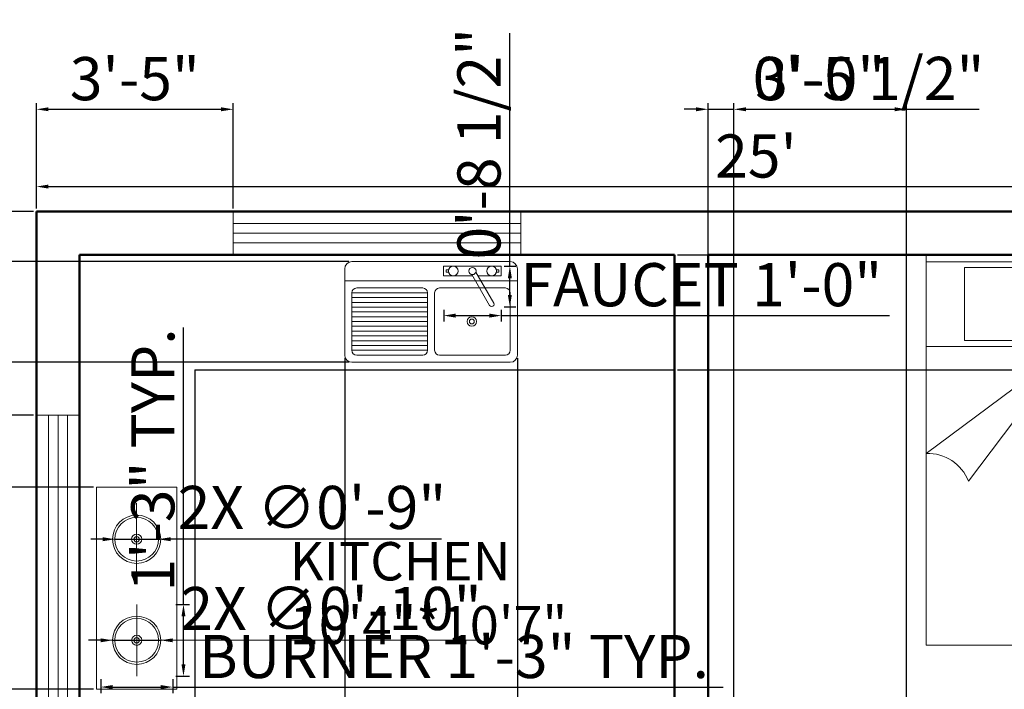
# Model space of a CAD drawing. Units: inches. Extents: x 2181 to 2717, y 1819 to 2296.
# Tile 4 of 5: x 2326 to 2531, y 2157 to 2296. Entities that reach past the tile are written whole.
import ezdxf

# ---------------------------------------------------------------- set-up
doc = ezdxf.new("R2010")
doc.units = ezdxf.units.IN
for name, color, linetype, lineweight in [('A-ANNO-DIMS', 2, 'Continuous', 13), ('A-AREA-IDEN', 7, 'Continuous', 25), ('A-EQPM', 9, 'Continuous', 18), ('A-FLOR-CASE', 32, 'Continuous', 25), ('A-FLOR-FIXT', 8, 'Continuous', 18), ('A-FURN', 8, 'Continuous', 18), ('A-GLAZ', 4, 'Continuous', 18), ('A-WALL', 7, 'Continuous', 50)]:
    doc.layers.add(name, color=color, linetype=linetype, lineweight=lineweight)
doc.styles.get("Standard").update_dxf_attribs({"font": 'arial.ttf'})
doc.dimstyles.new('ISO-25', dxfattribs={"dimtxt": 9, "dimasz": 2.5, "dimexe": 1.25, "dimexo": 0.625, "dimtad": 1, "dimlunit": 3, "dimtxsty": 'Standard', "dimcen": 2.5, "dimadec": 0, "dimazin": 0, "dimtfac": 1, "dimtmove": 0, "dimatfit": 3, "dimfxl": 1, "dimarcsym": 0})

# ---------------------------------------------------------------- blocks, each defined once
blk = doc.blocks.new('Faucet - kit sink top')
for p, q in [((-5.5, -0.75), (-5.5, -1.25)), ((-4.94278, -0.75), (-5.5, -0.75)), ((-5.5, -1.25), (-4.94278, -1.25)), ((-0.14775, -1.7441), (3.56698, -8.1782)), ((4.43301, -7.6782), (0.71828, -1.2441)), ((4.94278, -0.75), (5.5, -0.75)), ((5.5, -1.25), (4.94278, -1.25)), ((5.5, -0.75), (5.5, -1.25))]:
    blk.add_line(p, q)
blk.add_lwpolyline([(-0.00587, -2), (-6, -2), (-6, 0), (6, 0), (6, -2), (1.15195, -2)])
for centre, radius in [((-4, -1), 1), ((4, -1), 1), ((0, -1), 0.75)]:
    blk.add_circle(centre, radius)
blk.add_arc((4, -7.9282), 0.5, 210, 30)
blk = doc.blocks.new('*D8')
at = {"layer": 'A-ANNO-DIMS', "color": 0, "lineweight": -2, "transparency": 16777216}
for p, q in [((2329.35, 2256.83), (2329.35, 2262.67)), ((2629.35, 2256.83), (2629.35, 2262.67)), ((2331.85, 2261.42), (2626.85, 2261.42))]:
    blk.add_line(p, q, dxfattribs=at)
at = {"layer": 'A-ANNO-DIMS', "color": 0, "transparency": 16777216}
for points in [[(2331.85, 2261.84), (2331.85, 2261.01), (2329.35, 2261.42)], [(2626.85, 2261.84), (2626.85, 2261.01), (2629.35, 2261.42)]]:
    blk.add_solid(points, dxfattribs=at)
at = {"layer": 'Defpoints', "color": 0, "transparency": 16777216}
for p in [(2629.35, 2261.42), (2329.35, 2256.2), (2629.35, 2256.2)]:
    blk.add_point(p, dxfattribs=at)
at = {"layer": 'A-ANNO-DIMS', "color": 0, "transparency": 16777216, "insert": (2479.35, 2266.64), "char_height": 9, "attachment_point": 5}
blk.add_mtext("25'", dxfattribs=at)
blk = doc.blocks.new('WIN-60IN')
for p, q in [((0, 0), (0, 9)), ((60, 0), (60, 9)), ((60, 6.5), (0, 6.5)), ((60, 4.5), (0, 4.5)), ((60, 2.5), (0, 2.5))]:
    blk.add_line(p, q)
blk = doc.blocks.new('BED-QUEEN-PLAN')
for p, q in [((60.01, 81.47), (0, 81.47)), ((0, 81.47), (0, 80)), ((60.01, 80), (60.01, 81.47)), ((0.01, 0), (0.01, 80)), ((0.01, 80), (60.01, 80)), ((8.01, 78.8), (28.81, 78.8)), ((8.01, 63.6), (8.01, 78.8)), ((28.81, 78.8), (28.81, 63.6)), ((31.21, 78.8), (52.01, 78.8)), ((31.21, 63.6), (31.21, 78.8)), ((52.01, 78.8), (52.01, 63.6)), ((60.01, 80), (60.01, 0)), ((60.01, 62.35), (0.01, 62.35)), ((30.01, 62.35), (0.01, 40)), ((28.81, 63.6), (8.01, 63.6)), ((8.81, 34.19), (30.01, 62.35)), ((30.01, 62.35), (60.01, 40)), ((51.22, 34.19), (30.01, 62.35)), ((52.01, 63.6), (31.21, 63.6)), ((60.01, 0), (0.01, 0))]:
    blk.add_line(p, q)
for centre, start, end in [((0.34, 30.93), 21.0875, 92.0428), ((59.69, 30.93), 87.9572, 158.9125)]:
    blk.add_arc(centre, 9.08, start, end)
blk = doc.blocks.new('COOKTOP-BURNER')
for p in [(7.51, 15.01), (0, 7.51), (7.51, 0), (15.01, 7.51)]:
    blk.add_line(p, (7.51, 7.51))
for radius in [5.03, 4.55, 1.06, 0.557]:
    blk.add_circle((7.51, 7.51), radius)
blk = doc.blocks.new('*D21')
at = {"layer": 'A-ANNO-DIMS', "color": 0, "lineweight": -2, "transparency": 16777216}
for p, q in [((2342.73, 2158.61), (2342.73, 2155.73)), ((2357.74, 2158.61), (2357.74, 2155.73)), ((2345.23, 2156.98), (2355.24, 2156.98)), ((2357.74, 2156.98), (2472.54, 2156.98))]:
    blk.add_line(p, q, dxfattribs=at)
at = {"layer": 'A-ANNO-DIMS', "color": 0, "transparency": 16777216}
for points in [[(2345.23, 2157.4), (2345.23, 2156.56), (2342.73, 2156.98)], [(2355.24, 2157.4), (2355.24, 2156.56), (2357.74, 2156.98)]]:
    blk.add_solid(points, dxfattribs=at)
at = {"layer": 'Defpoints', "color": 0, "transparency": 16777216}
for p in [(2342.73, 2159.23), (2357.74, 2159.23), (2357.74, 2156.98)]:
    blk.add_point(p, dxfattribs=at)
at = {"layer": 'A-ANNO-DIMS', "color": 0, "transparency": 16777216, "insert": (2416.39, 2162.2), "char_height": 9, "attachment_point": 5}
blk.add_mtext('BURNER 1\'-3" TYP.', dxfattribs=at)
blk = doc.blocks.new('*D22')
at = {"layer": 'A-ANNO-DIMS', "color": 0, "lineweight": -2, "transparency": 16777216}
for p, q in [((2359.99, 2174.24), (2359.99, 2232.01)), ((2358.37, 2174.24), (2361.24, 2174.24)), ((2359.99, 2161.73), (2359.99, 2171.74)), ((2358.37, 2159.23), (2361.24, 2159.23))]:
    blk.add_line(p, q, dxfattribs=at)
at = {"layer": 'A-ANNO-DIMS', "color": 0, "transparency": 16777216}
for points in [[(2359.58, 2171.74), (2360.41, 2171.74), (2359.99, 2174.24)], [(2359.58, 2161.73), (2360.41, 2161.73), (2359.99, 2159.23)]]:
    blk.add_solid(points, dxfattribs=at)
at = {"layer": 'Defpoints', "color": 0, "transparency": 16777216}
for p in [(2357.74, 2174.24), (2359.99, 2174.24), (2357.74, 2159.23)]:
    blk.add_point(p, dxfattribs=at)
at = {"layer": 'A-ANNO-DIMS', "color": 0, "transparency": 16777216, "insert": (2354.77, 2204.37), "char_height": 9, "attachment_point": 5, "rotation": 90}
blk.add_mtext('1\'-3" TYP.', dxfattribs=at)
blk = doc.blocks.new('*D23')
at = {"layer": 'A-ANNO-DIMS', "color": 0, "lineweight": -2, "transparency": 16777216}
for p, q in [((2414.24, 2235.68), (2414.24, 2233.25)), ((2426.24, 2235.68), (2426.24, 2233.25)), ((2416.74, 2234.5), (2423.74, 2234.5)), ((2426.24, 2234.5), (2507.19, 2234.5))]:
    blk.add_line(p, q, dxfattribs=at)
at = {"layer": 'A-ANNO-DIMS', "color": 0, "transparency": 16777216}
for points in [[(2416.74, 2234.92), (2416.74, 2234.08), (2414.24, 2234.5)], [(2423.74, 2234.92), (2423.74, 2234.08), (2426.24, 2234.5)]]:
    blk.add_solid(points, dxfattribs=at)
at = {"layer": 'Defpoints', "color": 0, "transparency": 16777216}
for p in [(2414.24, 2236.3), (2426.24, 2236.3), (2426.24, 2234.5)]:
    blk.add_point(p, dxfattribs=at)
at = {"layer": 'A-ANNO-DIMS', "color": 0, "transparency": 16777216, "insert": (2467.96, 2239.78), "char_height": 9, "attachment_point": 5}
blk.add_mtext('FAUCET 1\'-0"', dxfattribs=at)
blk = doc.blocks.new('*D24')
at = {"layer": 'A-ANNO-DIMS', "color": 0, "lineweight": -2, "transparency": 16777216}
for p, q in [((2428.04, 2244.8), (2428.04, 2293.45)), ((2426.86, 2244.8), (2429.29, 2244.8)), ((2428.04, 2238.8), (2428.04, 2242.3)), ((2426.86, 2236.3), (2429.29, 2236.3))]:
    blk.add_line(p, q, dxfattribs=at)
at = {"layer": 'A-ANNO-DIMS', "color": 0, "transparency": 16777216}
for points in [[(2427.62, 2242.3), (2428.45, 2242.3), (2428.04, 2244.8)], [(2427.62, 2238.8), (2428.45, 2238.8), (2428.04, 2236.3)]]:
    blk.add_solid(points, dxfattribs=at)
at = {"layer": 'Defpoints', "color": 0, "transparency": 16777216}
for p in [(2426.24, 2244.8), (2428.04, 2244.8), (2426.24, 2236.3)]:
    blk.add_point(p, dxfattribs=at)
at = {"layer": 'A-ANNO-DIMS', "color": 0, "transparency": 16777216, "insert": (2422.76, 2270.37), "char_height": 9, "attachment_point": 5, "rotation": 90}
blk.add_mtext('0\'-8 1/2"', dxfattribs=at)
blk = doc.blocks.new('*D25')
at = {"layer": 'A-ANNO-DIMS', "color": 0, "lineweight": -2, "transparency": 16777216}
for p, q in [((2329.35, 2256.83), (2329.35, 2278.8)), ((2370.35, 2256.83), (2370.35, 2278.8)), ((2331.85, 2277.55), (2367.85, 2277.55))]:
    blk.add_line(p, q, dxfattribs=at)
at = {"layer": 'A-ANNO-DIMS', "color": 0, "transparency": 16777216}
for points in [[(2331.85, 2277.97), (2331.85, 2277.14), (2329.35, 2277.55)], [(2367.85, 2277.97), (2367.85, 2277.14), (2370.35, 2277.55)]]:
    blk.add_solid(points, dxfattribs=at)
at = {"layer": 'Defpoints', "color": 0, "transparency": 16777216}
for p in [(2370.35, 2277.55), (2329.35, 2256.2), (2370.35, 2256.2)]:
    blk.add_point(p, dxfattribs=at)
at = {"layer": 'A-ANNO-DIMS', "color": 0, "transparency": 16777216, "insert": (2349.85, 2282.78), "char_height": 9, "attachment_point": 5}
blk.add_mtext('3\'-5"', dxfattribs=at)
blk = doc.blocks.new('*D26')
at = {"layer": 'A-ANNO-DIMS', "color": 0, "lineweight": -2, "transparency": 16777216}
for p, q in [((2328.72, 2256.2), (2306.75, 2256.2)), ((2308, 2253.7), (2308, 2216.2)), ((2328.72, 2213.7), (2306.75, 2213.7)), ((2308, 2213.7), (2308, 2165.07))]:
    blk.add_line(p, q, dxfattribs=at)
at = {"layer": 'A-ANNO-DIMS', "color": 0, "transparency": 16777216}
for points in [[(2307.58, 2253.7), (2308.41, 2253.7), (2308, 2256.2)], [(2307.58, 2216.2), (2308.41, 2216.2), (2308, 2213.7)]]:
    blk.add_solid(points, dxfattribs=at)
at = {"layer": 'Defpoints', "color": 0, "transparency": 16777216}
for p in [(2329.35, 2256.2), (2308, 2213.7), (2329.35, 2213.7)]:
    blk.add_point(p, dxfattribs=at)
at = {"layer": 'A-ANNO-DIMS', "color": 0, "transparency": 16777216, "insert": (2302.71, 2188.13), "char_height": 9, "attachment_point": 5, "rotation": 90}
blk.add_mtext('3\'-6 1/2"', dxfattribs=at)
blk = doc.blocks.new('*D40')
at = {"layer": 'A-ANNO-DIMS', "color": 0, "lineweight": -2, "transparency": 16777216}
for p, q in [((2474.75, 2120.83), (2474.75, 2278.8)), ((2510.75, 2120.83), (2510.75, 2278.8)), ((2477.25, 2277.55), (2508.25, 2277.55))]:
    blk.add_line(p, q, dxfattribs=at)
at = {"layer": 'A-ANNO-DIMS', "color": 0, "transparency": 16777216}
for points in [[(2477.25, 2277.97), (2477.25, 2277.14), (2474.75, 2277.55)], [(2508.25, 2277.97), (2508.25, 2277.14), (2510.75, 2277.55)]]:
    blk.add_solid(points, dxfattribs=at)
at = {"layer": 'Defpoints', "color": 0, "transparency": 16777216}
for p in [(2510.75, 2277.55), (2474.75, 2120.2), (2510.75, 2120.2)]:
    blk.add_point(p, dxfattribs=at)
at = {"layer": 'A-ANNO-DIMS', "color": 0, "transparency": 16777216, "insert": (2492.75, 2282.78), "char_height": 9, "attachment_point": 5}
blk.add_mtext('3\'-0"', dxfattribs=at)
blk = doc.blocks.new('*D42')
at = {"layer": 'A-ANNO-DIMS', "color": 0, "lineweight": -2, "transparency": 16777216}
for p, q in [((2701.7, 2247.2), (2701.7, 2275.03)), ((2462.97, 2247.2), (2702.95, 2247.2)), ((2701.7, 2225.7), (2701.7, 2244.7)), ((2462.97, 2223.2), (2702.95, 2223.2))]:
    blk.add_line(p, q, dxfattribs=at)
at = {"layer": 'A-ANNO-DIMS', "color": 0, "transparency": 16777216}
for points in [[(2701.28, 2244.7), (2702.11, 2244.7), (2701.7, 2247.2)], [(2701.28, 2225.7), (2702.11, 2225.7), (2701.7, 2223.2)]]:
    blk.add_solid(points, dxfattribs=at)
at = {"layer": 'Defpoints', "color": 0, "transparency": 16777216}
for p in [(2462.35, 2247.2), (2701.7, 2247.2), (2462.35, 2223.2)]:
    blk.add_point(p, dxfattribs=at)
at = {"layer": 'A-ANNO-DIMS', "color": 0, "transparency": 16777216, "insert": (2696.48, 2262.37), "char_height": 9, "attachment_point": 5, "rotation": 90}
blk.add_mtext('2\'-0"', dxfattribs=at)
blk = doc.blocks.new('*D43')
at = {"layer": 'A-ANNO-DIMS', "color": 0, "lineweight": -2, "transparency": 16777216}
for p, q in [((2393.61, 2225.64), (2393.61, 1825.6)), ((2429.61, 2225.64), (2429.61, 1825.6)), ((2396.11, 1826.85), (2427.11, 1826.85))]:
    blk.add_line(p, q, dxfattribs=at)
at = {"layer": 'A-ANNO-DIMS', "color": 0, "transparency": 16777216}
for points in [[(2396.11, 1827.27), (2396.11, 1826.44), (2393.61, 1826.85)], [(2427.11, 1827.27), (2427.11, 1826.44), (2429.61, 1826.85)]]:
    blk.add_solid(points, dxfattribs=at)
at = {"layer": 'Defpoints', "color": 0, "transparency": 16777216}
for p in [(2393.61, 2226.26), (2429.61, 2226.26), (2429.61, 1826.85)]:
    blk.add_point(p, dxfattribs=at)
at = {"layer": 'A-ANNO-DIMS', "color": 0, "transparency": 16777216, "insert": (2411.61, 1832.08), "char_height": 9, "attachment_point": 5}
blk.add_mtext('3\'-0"', dxfattribs=at)
blk = doc.blocks.new('*D44')
at = {"layer": 'A-ANNO-DIMS', "color": 0, "lineweight": -2, "transparency": 16777216}
for p, q in [((2308, 2245.76), (2308, 2272.59)), ((2394.49, 2245.76), (2306.75, 2245.76)), ((2308, 2227.26), (2308, 2243.26)), ((2394.49, 2224.76), (2306.75, 2224.76))]:
    blk.add_line(p, q, dxfattribs=at)
at = {"layer": 'A-ANNO-DIMS', "color": 0, "transparency": 16777216}
for points in [[(2307.58, 2243.26), (2308.41, 2243.26), (2308, 2245.76)], [(2307.58, 2227.26), (2308.41, 2227.26), (2308, 2224.76)]]:
    blk.add_solid(points, dxfattribs=at)
at = {"layer": 'Defpoints', "color": 0, "transparency": 16777216}
for p in [(2308, 2245.76), (2395.11, 2245.76), (2395.11, 2224.76)]:
    blk.add_point(p, dxfattribs=at)
at = {"layer": 'A-ANNO-DIMS', "color": 0, "transparency": 16777216, "insert": (2302.78, 2260.43), "char_height": 9, "attachment_point": 5, "rotation": 90}
blk.add_mtext('1\'-9"', dxfattribs=at)
blk = doc.blocks.new('*D45')
at = {"layer": 'A-ANNO-DIMS', "color": 0, "lineweight": -2, "transparency": 16777216}
for p, q in [((2429.61, 2225.64), (2429.61, 1825.6)), ((2462.35, 2222.58), (2462.35, 1825.6)), ((2432.11, 1826.85), (2459.85, 1826.85)), ((2462.35, 1826.85), (2511.15, 1826.85))]:
    blk.add_line(p, q, dxfattribs=at)
at = {"layer": 'A-ANNO-DIMS', "color": 0, "transparency": 16777216}
for points in [[(2432.11, 1827.27), (2432.11, 1826.44), (2429.61, 1826.85)], [(2459.85, 1827.27), (2459.85, 1826.44), (2462.35, 1826.85)]]:
    blk.add_solid(points, dxfattribs=at)
at = {"layer": 'Defpoints', "color": 0, "transparency": 16777216}
for p in [(2429.61, 2226.26), (2462.35, 2223.2), (2462.35, 1826.85)]:
    blk.add_point(p, dxfattribs=at)
at = {"layer": 'A-ANNO-DIMS', "color": 0, "transparency": 16777216, "insert": (2488, 1832.13), "char_height": 9, "attachment_point": 5}
blk.add_mtext('2\'-8 1/2"', dxfattribs=at)
blk = doc.blocks.new('*D46')
at = {"layer": 'A-ANNO-DIMS', "color": 0, "lineweight": -2, "transparency": 16777216}
for p, q in [((2341.24, 2198.7), (2306.75, 2198.7)), ((2308, 2159.01), (2308, 2196.2)), ((2341.24, 2156.51), (2306.75, 2156.51))]:
    blk.add_line(p, q, dxfattribs=at)
at = {"layer": 'A-ANNO-DIMS', "color": 0, "transparency": 16777216}
for points in [[(2307.58, 2196.2), (2308.41, 2196.2), (2308, 2198.7)], [(2307.58, 2159.01), (2308.41, 2159.01), (2308, 2156.51)]]:
    blk.add_solid(points, dxfattribs=at)
at = {"layer": 'Defpoints', "color": 0, "transparency": 16777216}
for p in [(2308, 2198.7), (2341.86, 2198.7), (2341.86, 2156.51)]:
    blk.add_point(p, dxfattribs=at)
at = {"layer": 'A-ANNO-DIMS', "color": 0, "transparency": 16777216, "insert": (2302.77, 2177.61), "char_height": 9, "attachment_point": 5, "rotation": 90}
blk.add_mtext('3\'-6"', dxfattribs=at)
blk = doc.blocks.new('*D48')
at = {"layer": 'A-ANNO-DIMS', "color": 0, "lineweight": -2, "transparency": 16777216}
for p, q in [((2308, 2156.51), (2308, 2205.15)), ((2341.24, 2156.51), (2306.75, 2156.51)), ((2308, 2122.7), (2308, 2154.01)), ((2337.72, 2120.2), (2306.75, 2120.2))]:
    blk.add_line(p, q, dxfattribs=at)
at = {"layer": 'A-ANNO-DIMS', "color": 0, "transparency": 16777216}
for points in [[(2307.58, 2154.01), (2308.41, 2154.01), (2308, 2156.51)], [(2307.58, 2122.7), (2308.41, 2122.7), (2308, 2120.2)]]:
    blk.add_solid(points, dxfattribs=at)
at = {"layer": 'Defpoints', "color": 0, "transparency": 16777216}
for p in [(2308, 2156.51), (2341.86, 2156.51), (2338.35, 2120.2)]:
    blk.add_point(p, dxfattribs=at)
at = {"layer": 'A-ANNO-DIMS', "color": 0, "transparency": 16777216, "insert": (2302.71, 2182.08), "char_height": 9, "attachment_point": 5, "rotation": 90}
blk.add_mtext('3\'-0 1/2"', dxfattribs=at)
blk = doc.blocks.new('*D61')
at = {"layer": 'A-ANNO-DIMS', "color": 0, "lineweight": -2, "transparency": 16777216}
for p, q in [((2469.35, 2120.83), (2469.35, 2278.8)), ((2474.75, 2120.83), (2474.75, 2278.8)), ((2466.85, 2277.55), (2464.35, 2277.55)), ((2469.35, 2277.55), (2474.75, 2277.55)), ((2477.25, 2277.55), (2525.9, 2277.55))]:
    blk.add_line(p, q, dxfattribs=at)
at = {"layer": 'A-ANNO-DIMS', "color": 0, "transparency": 16777216}
for points in [[(2466.85, 2277.97), (2466.85, 2277.14), (2469.35, 2277.55)], [(2477.25, 2277.97), (2477.25, 2277.14), (2474.75, 2277.55)]]:
    blk.add_solid(points, dxfattribs=at)
at = {"layer": 'Defpoints', "color": 0, "transparency": 16777216}
for p in [(2474.75, 2277.55), (2469.35, 2120.2), (2474.75, 2120.2)]:
    blk.add_point(p, dxfattribs=at)
at = {"layer": 'A-ANNO-DIMS', "color": 0, "transparency": 16777216, "insert": (2502.82, 2282.83), "char_height": 9, "attachment_point": 5}
blk.add_mtext('0\'-5 1/2"', dxfattribs=at)
blk = doc.blocks.new('*D63')
at = {"layer": 'A-ANNO-DIMS', "color": 0, "lineweight": -2, "transparency": 16777216}
for p, q in [((2342.7, 2166.74), (2340.2, 2166.74)), ((2345.2, 2166.74), (2355.27, 2166.74)), ((2421.24, 2166.73), (2357.77, 2166.74))]:
    blk.add_line(p, q, dxfattribs=at)
at = {"layer": 'A-ANNO-DIMS', "color": 0, "transparency": 16777216}
for points in [[(2342.7, 2167.15), (2342.7, 2166.32), (2345.2, 2166.74)], [(2357.77, 2167.15), (2357.77, 2166.32), (2355.27, 2166.74)]]:
    blk.add_solid(points, dxfattribs=at)
at = {"layer": 'Defpoints', "color": 0, "transparency": 16777216}
for p in [(2345.2, 2166.74), (2355.27, 2166.74)]:
    blk.add_point(p, dxfattribs=at)
at = {"layer": 'A-ANNO-DIMS', "color": 0, "transparency": 16777216, "insert": (2390.75, 2172.21), "char_height": 9, "attachment_point": 5, "rotation": 359.9974}
blk.add_mtext('2X ∅0\'-10"', dxfattribs=at)
blk = doc.blocks.new('*D64')
at = {"layer": 'A-ANNO-DIMS', "color": 0, "lineweight": -2, "transparency": 16777216}
for p, q in [((2343.18, 2187.83), (2340.68, 2187.83)), ((2345.68, 2187.83), (2354.79, 2187.83)), ((2413.77, 2187.83), (2357.29, 2187.83))]:
    blk.add_line(p, q, dxfattribs=at)
at = {"layer": 'A-ANNO-DIMS', "color": 0, "transparency": 16777216}
for points in [[(2343.18, 2188.25), (2343.18, 2187.42), (2345.68, 2187.83)], [(2357.29, 2188.25), (2357.29, 2187.42), (2354.79, 2187.83)]]:
    blk.add_solid(points, dxfattribs=at)
at = {"layer": 'Defpoints', "color": 0, "transparency": 16777216}
for p in [(2345.68, 2187.83), (2354.79, 2187.83)]:
    blk.add_point(p, dxfattribs=at)
at = {"layer": 'A-ANNO-DIMS', "color": 0, "transparency": 16777216, "insert": (2386.78, 2193.3), "char_height": 9, "attachment_point": 5, "rotation": 359.9974}
blk.add_mtext('2X ∅0\'-9"', dxfattribs=at)

msp = doc.modelspace()

# ---------------------------------------------------------------- linework, layer by layer
at = {"layer": 'A-EQPM'}
msp.add_lwpolyline([(2341.861, 2198.704), (2358.609, 2198.704), (2358.609, 2156.51), (2341.861, 2156.51)], close=True, dxfattribs=at)
at = {"layer": 'A-FLOR-CASE'}
for q in [(2362.346, 2120.205), (2462.346, 2223.205)]:
    msp.add_line((2362.346, 2223.205), q, dxfattribs=at)
at = {"layer": 'A-FLOR-FIXT'}
for p, q in [((2393.61, 2241.763), (2429.61, 2241.763)), ((2410.86, 2227.263), (2410.86, 2239.263)), ((2412.36, 2239.263), (2412.36, 2227.263)), ((2396.11, 2226.263), (2409.86, 2226.263))]:
    msp.add_line(p, q, dxfattribs=at)
for points in [[(2395.11, 2245.763), (2428.11, 2245.763)], [(2393.61, 2226.263), (2393.61, 2244.263)], [(2429.61, 2244.263), (2429.61, 2226.263)], [(2396.11, 2240.263), (2409.86, 2240.263)], [(2413.36, 2240.263), (2427.11, 2240.263)], [(2395.11, 2227.263), (2395.11, 2239.263)], [(2395.11, 2239.263), (2410.86, 2239.263)], [(2395.11, 2238.263), (2410.86, 2238.263)], [(2428.11, 2239.263), (2428.11, 2227.263)], [(2395.11, 2237.263), (2410.86, 2237.263)], [(2395.11, 2236.263), (2410.86, 2236.263)], [(2395.11, 2235.263), (2410.86, 2235.263)], [(2395.11, 2234.263), (2410.86, 2234.263)], [(2395.11, 2233.263), (2410.86, 2233.263)], [(2395.11, 2232.263), (2410.86, 2232.263)], [(2395.11, 2231.263), (2410.86, 2231.263)], [(2395.11, 2230.263), (2410.86, 2230.263)], [(2395.11, 2229.263), (2410.86, 2229.263)], [(2395.11, 2228.263), (2410.86, 2228.263)], [(2395.11, 2227.263), (2410.86, 2227.263)], [(2427.11, 2226.263), (2413.36, 2226.263)], [(2428.11, 2224.763), (2395.11, 2224.763)]]:
    msp.add_lwpolyline(points, dxfattribs=at)
for radius in [1, 0.5]:
    msp.add_circle((2420.11, 2233.263), radius, dxfattribs=at)
for centre, radius, start, end in [((2395.11, 2244.263), 1.5, 90, 180), ((2428.11, 2244.263), 1.5, 0, 90), ((2396.11, 2239.263), 1, 90, 180), ((2409.86, 2239.263), 1, 0, 90), ((2413.36, 2239.263), 1, 90, 180), ((2427.11, 2239.263), 1, 0, 90), ((2396.11, 2227.263), 1, 180, 270), ((2409.86, 2227.263), 1, 270, 0), ((2413.36, 2227.263), 1, 180, 270), ((2427.11, 2227.263), 1, 270, 0), ((2395.11, 2226.263), 1.5, 180, 270), ((2428.11, 2226.263), 1.5, 270, 0)]:
    msp.add_arc(centre, radius, start, end, dxfattribs=at)
at = {"layer": 'A-WALL'}
for p, q in [((2329.346, 2256.205), (2629.346, 2256.205)), ((2329.346, 2256.205), (2329.346, 1872.205)), ((2338.346, 2247.205), (2462.346, 2247.205)), ((2338.346, 2247.205), (2338.346, 2120.205)), ((2462.346, 2247.205), (2462.346, 2120.205)), ((2469.346, 2247.205), (2469.346, 2120.205)), ((2469.346, 2247.205), (2620.346, 2247.205))]:
    msp.add_line(p, q, dxfattribs=at)

# ---------------------------------------------------------------- block references
at = {"layer": 'A-EQPM', "rotation": 180}
msp.add_blockref('COOKTOP-BURNER', (2357.741, 2195.34), dxfattribs=at)
at = {"layer": 'A-EQPM'}
msp.add_blockref('COOKTOP-BURNER', (2342.729, 2159.231), dxfattribs=at)
at = {"layer": 'A-FLOR-FIXT'}
msp.add_blockref('Faucet - kit sink top', (2420.235, 2244.8), dxfattribs=at)
at = {"layer": 'A-FURN'}
msp.add_blockref('BED-QUEEN-PLAN', (2514.834, 2165.732), dxfattribs=at)
at = {"layer": 'A-GLAZ'}
msp.add_blockref('WIN-60IN', (2370.346, 2247.205), dxfattribs=at)
at = {"layer": 'A-GLAZ', "rotation": 89.99999999999747}
msp.add_blockref('WIN-60IN', (2338.346, 2153.704), dxfattribs=at)

# ---------------------------------------------------------------- texts
at = {"layer": 'A-AREA-IDEN', "insert": (2382.148, 2187.238), "char_height": 8, "attachment_point": 1}
msp.add_mtext_dynamic_manual_height_columns('KITCHEN\\P10\'4"*10\'7"', width=56.09608, gutter_width=12.5, heights=[0], dxfattribs=at)

# ---------------------------------------------------------------- dimensions: what is measured, and where the dimension line sits
at = {"layer": 'A-ANNO-DIMS'}
for base, p1, p2, picture, middle in [((2474.75, 2277.555), (2469.346, 2120.205), (2474.75, 2120.205), '*D61', (2502.823, 2282.833)), ((2370.346, 2277.555), (2329.346, 2256.205), (2370.346, 2256.205), '*D25', (2349.846, 2282.778)), ((2510.745, 2277.555), (2474.75, 2120.205), (2510.745, 2120.205), '*D40', (2492.748, 2282.778)), ((2429.61, 1826.855), (2393.61, 2226.263), (2429.61, 2226.263), '*D43', (2411.61, 1832.078)), ((2462.346, 1826.855), (2429.61, 2226.263), (2462.346, 2223.205), '*D45', (2487.996, 1832.133))]:
    dim = msp.add_linear_dim(base=base, p1=p1, p2=p2, dimstyle='ISO-25', override={"dimdec": 1, "dimlfac": 1, "dimrnd": 0, "dimzin": 1, "dimdsep": 46, "dimlunit": 4, "dimfrac": 2}, dxfattribs=at)
    dim.commit()
    dim.dimension.update_dxf_attribs({"geometry": picture, "text_midpoint": middle})
for base, p1, p2, picture, middle in [((2428.035, 2244.8), (2426.235, 2236.301), (2426.235, 2244.8), '*D24', (2422.757, 2270.373)), ((2701.696, 2247.205), (2462.346, 2223.205), (2462.346, 2247.205), '*D42', (2696.476, 2262.368)), ((2307.996, 2245.763), (2395.11, 2224.763), (2395.11, 2245.763), '*D44', (2302.776, 2260.426)), ((2307.996, 2213.705), (2329.346, 2256.205), (2329.346, 2213.705), '*D26', (2302.715, 2188.135)), ((2307.996, 2156.51), (2338.346, 2120.205), (2341.861, 2156.51), '*D48', (2302.715, 2182.08)), ((2307.996, 2198.704), (2341.861, 2156.51), (2341.861, 2198.704), '*D46', (2302.773, 2177.607))]:
    dim = msp.add_linear_dim(base=base, p1=p1, p2=p2, angle=90, dimstyle='ISO-25', override={"dimdec": 1, "dimlfac": 1, "dimrnd": 0, "dimzin": 1, "dimdsep": 46, "dimlunit": 4, "dimfrac": 2}, dxfattribs=at)
    dim.commit()
    dim.dimension.update_dxf_attribs({"geometry": picture, "text_midpoint": middle})
dim = msp.add_linear_dim(base=(2629.346, 2261.425), p1=(2329.346, 2256.205), p2=(2629.346, 2256.205), dimstyle='ISO-25', override={"dimclrd": 0, "dimclre": 0, "dimclrt": 0}, dxfattribs=at)
dim.commit()
dim.dimension.update_dxf_attribs({"geometry": '*D8', "text_midpoint": (2479.346, 2261.425), "dimtype": 160})
for base, p1, p2, text, picture, middle in [((2426.235, 2234.501), (2414.235, 2236.301), (2426.235, 2236.301), 'FAUCET <>', '*D23', (2467.96, 2239.78)), ((2357.741, 2156.979), (2342.729, 2159.231), (2357.741, 2159.231), 'BURNER <> TYP.', '*D21', (2416.388, 2162.203))]:
    dim = msp.add_linear_dim(base=base, p1=p1, p2=p2, text=text, dimstyle='ISO-25', override={"dimdec": 1, "dimlfac": 1, "dimrnd": 0, "dimzin": 1, "dimdsep": 46, "dimlunit": 4, "dimfrac": 2}, dxfattribs=at)
    dim.commit()
    dim.dimension.update_dxf_attribs({"geometry": picture, "text_midpoint": middle})
dim = msp.add_linear_dim(base=(2359.993, 2174.243), p1=(2357.741, 2159.231), p2=(2357.741, 2174.243), angle=90, text='<> TYP.', dimstyle='ISO-25', override={"dimdec": 1, "dimlfac": 1, "dimrnd": 0, "dimzin": 1, "dimdsep": 46, "dimlunit": 4, "dimfrac": 2}, dxfattribs=at)
dim.commit()
dim.dimension.update_dxf_attribs({"geometry": '*D22', "text_midpoint": (2354.77, 2204.374)})
for p1, p2, picture, middle in [((2345.682, 2187.834), (2354.788, 2187.834), '*D64', (2386.778, 2187.833)), ((2345.203, 2166.737), (2355.267, 2166.737), '*D63', (2390.753, 2166.735))]:
    dim = msp.add_diameter_dim_2p(p1=p1, p2=p2, text='2X <>', dimstyle='ISO-25', override={"dimdec": 1, "dimlfac": 1, "dimrnd": 0, "dimzin": 1, "dimdsep": 46, "dimlunit": 4, "dimfrac": 2}, dxfattribs=at)
    dim.commit()
    dim.dimension.update_dxf_attribs({"geometry": picture, "text_midpoint": middle})

doc.saveas('drawing.dxf')
